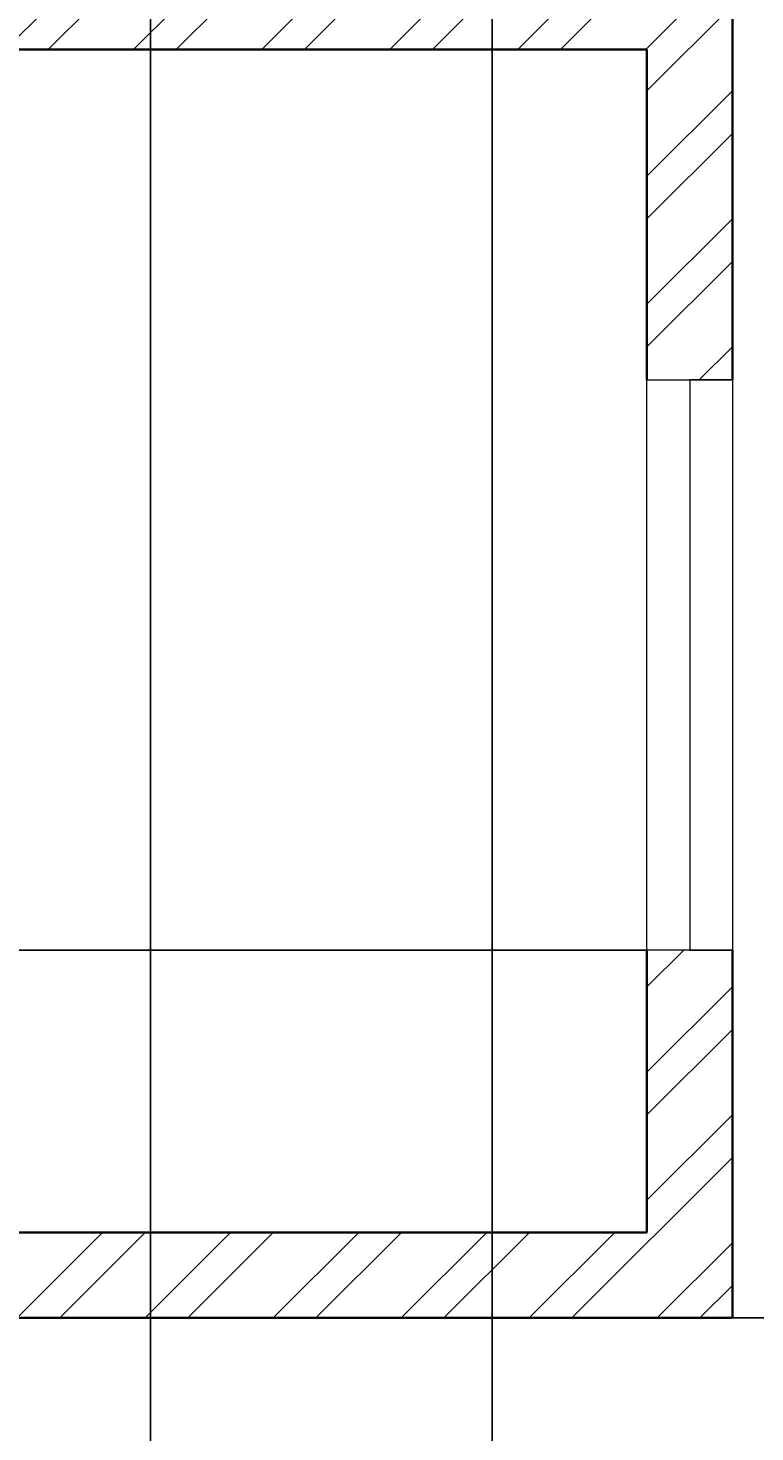
# Model space of a CAD drawing. Units: inches. Extents: x 1748 to 2382, y 1346 to 2284.
# Tile 14 of 26: x 2223 to 2300, y 1456 to 1604. Entities that reach past the tile are written whole.
import ezdxf

# ---------------------------------------------------------------- set-up
doc = ezdxf.new("R2010")
doc.units = ezdxf.units.IN
for name, color, linetype, lineweight in [('A-ANNO-DIMS', 2, 'Continuous', 18), ('A-GLAZ', 191, 'Continuous', 18), ('A-WALL', 7, 'Continuous', 35), ('A-WALL-PATT', 9, 'Continuous', 13)]:
    doc.layers.add(name, color=color, linetype=linetype, lineweight=lineweight)
doc.styles.get("Standard").update_dxf_attribs({"font": 'arial.ttf'})
doc.dimstyles.get("Standard").update_dxf_attribs({"dimtxt": 0.18, "dimasz": 0.18, "dimexe": 0.18, "dimexo": 0.0625, "dimgap": 0.09, "dimtad": 0, "dimtih": 1, "dimtoh": 1, "dimdec": 4, "dimzin": 0, "dimdsep": 46, "dimtxsty": 'Standard', "dimcen": 0.09, "dimadec": 0, "dimazin": 0, "dimtfac": 1, "dimtdec": 4, "dimtofl": 0, "dimtmove": 0, "dimatfit": 3, "dimfxl": 1, "dimtolj": 1, "dimtzin": 0, "dimarcsym": 0})

# ---------------------------------------------------------------- blocks, each defined once
blk = doc.blocks.new('*D35')
at = {"layer": 'A-ANNO-DIMS', "color": 0, "lineweight": -2, "transparency": 16777216}
for p, q in [((2297.52, 2232.85), (2339.54, 2232.85)), ((2339.36, 2232.67), (2339.36, 1850.53)), ((2339.36, 1468.03), (2339.36, 1850.17)), ((2297.52, 1467.85), (2339.54, 1467.85))]:
    blk.add_line(p, q, dxfattribs=at)
at = {"layer": 'A-ANNO-DIMS', "color": 0, "transparency": 16777216}
for points in [[(2339.33, 2232.67), (2339.39, 2232.67), (2339.36, 2232.85)], [(2339.33, 1468.03), (2339.39, 1468.03), (2339.36, 1467.85)]]:
    blk.add_solid(points, dxfattribs=at)
at = {"layer": 'Defpoints', "color": 0, "transparency": 16777216}
for p in [(2297.46, 2232.85), (2339.36, 2232.85), (2297.46, 1467.85)]:
    blk.add_point(p, dxfattribs=at)
at = {"layer": 'A-ANNO-DIMS', "color": 0, "transparency": 16777216, "insert": (2339.36, 1850.35), "char_height": 0.18, "attachment_point": 5}
blk.add_mtext('\\A1;765', dxfattribs=at)
blk = doc.blocks.new('*D49')
at = {"layer": 'A-ANNO-DIMS', "color": 0, "lineweight": -2, "transparency": 16777216}
for p, q in [((2236.23, 1913.29), (2236.23, 1360.47)), ((2272.19, 1913.29), (2272.19, 1360.47)), ((2236.41, 1360.65), (2253.82, 1360.65)), ((2272.01, 1360.65), (2254.61, 1360.65))]:
    blk.add_line(p, q, dxfattribs=at)
at = {"layer": 'A-ANNO-DIMS', "color": 0, "transparency": 16777216}
for points in [[(2236.41, 1360.68), (2236.41, 1360.62), (2236.23, 1360.65)], [(2272.01, 1360.68), (2272.01, 1360.62), (2272.19, 1360.65)]]:
    blk.add_solid(points, dxfattribs=at)
at = {"layer": 'Defpoints', "color": 0, "transparency": 16777216}
for p in [(2236.23, 1913.35), (2272.19, 1913.35), (2272.19, 1360.65)]:
    blk.add_point(p, dxfattribs=at)
at = {"layer": 'A-ANNO-DIMS', "color": 0, "transparency": 16777216, "insert": (2254.21, 1360.65), "char_height": 0.18, "attachment_point": 5}
blk.add_mtext('\\A1;35.96', dxfattribs=at)
blk = doc.blocks.new('*D54')
at = {"layer": 'A-ANNO-DIMS', "color": 0, "lineweight": -2, "transparency": 16777216}
for p, q in [((2288.4, 1506.57), (1779.88, 1506.57)), ((1780.06, 1506.39), (1780.06, 1491.89)), ((1780.06, 1477.03), (1780.06, 1491.53)), ((2288.4, 1476.85), (1779.88, 1476.85))]:
    blk.add_line(p, q, dxfattribs=at)
at = {"layer": 'A-ANNO-DIMS', "color": 0, "transparency": 16777216}
for points in [[(1780.03, 1506.39), (1780.09, 1506.39), (1780.06, 1506.57)], [(1780.03, 1477.03), (1780.09, 1477.03), (1780.06, 1476.85)]]:
    blk.add_solid(points, dxfattribs=at)
at = {"layer": 'Defpoints', "color": 0, "transparency": 16777216}
for p in [(1780.06, 1506.57), (2288.46, 1506.57), (2288.46, 1476.85)]:
    blk.add_point(p, dxfattribs=at)
at = {"layer": 'A-ANNO-DIMS', "color": 0, "transparency": 16777216, "insert": (1780.06, 1491.71), "char_height": 0.18, "attachment_point": 5}
blk.add_mtext('\\A1;29.716', dxfattribs=at)

msp = doc.modelspace()

# ---------------------------------------------------------------- hatches: boundary and pattern name
at = {"layer": 'A-WALL-PATT'}
h = msp.add_hatch(dxfattribs=at)
h.set_pattern_fill('ANSI32', color=256)
h.paths.add_polyline_path([(1919.6777, 1476.8497), (1900.6426, 1476.8497), (1900.6426, 1522.0826), (1898.3926, 1522.0826), (1896.1426, 1522.0826), (1896.1426, 1476.8497), (1857.1426, 1476.8497), (1857.1426, 1467.8497), (1896.1426, 1467.8497), (1919.6777, 1467.8497), (1919.6777, 1472.3497)])
h.paths.add_polyline_path([(2018.7873, 1472.3497), (2018.7873, 1476.8497), (2010.9607, 1476.8497), (2010.9607, 1560.8497), (2034.9607, 1560.8497), (2034.9607, 1565.3497), (2006.4607, 1565.3497), (2006.4607, 1476.8497), (1955.6777, 1476.8497), (1955.6777, 1467.8497), (2018.7873, 1467.8497)])
h.paths.add_polyline_path([(2152.3354, 1472.3497), (2152.3354, 1476.8497), (2115.9607, 1476.8497), (2115.9607, 1565.3497), (2109.2204, 1565.3497), (2109.2204, 1563.0997), (2109.2204, 1560.8497), (2111.4607, 1560.8497), (2111.4607, 1476.8497), (2095.3617, 1476.8497), (2095.3617, 1467.8497), (2152.3354, 1467.8497)])
h.paths.add_polyline_path([(2071.3617, 1476.8497), (2063.4607, 1476.8497), (2063.4607, 1560.8497), (2090.1865, 1560.8497), (2090.1865, 1565.3497), (2063.4607, 1565.3497), (2063.4607, 1572.5485), (2061.2107, 1572.5485), (2058.9607, 1572.5485), (2058.9607, 1565.3497), (2055.6281, 1565.3497), (2055.6281, 1560.8497), (2058.9607, 1560.8497), (2058.9607, 1476.8497), (2042.7873, 1476.8497), (2042.7873, 1467.8497), (2071.3617, 1467.8497), (2071.3617, 1472.3497)])
h.paths.add_polyline_path([(2297.4607, 1506.5652), (2288.4607, 1506.5652), (2288.4607, 1476.8497), (2212.3354, 1476.8497), (2212.3354, 1467.8497), (2297.4607, 1467.8497)])
h.paths.add_polyline_path([(2297.4607, 1645.3038), (2288.4607, 1645.3038), (2288.4607, 1605.8497), (2058.9607, 1605.8497), (2058.9607, 1600.1857), (2061.2107, 1600.1857), (2063.4607, 1600.1857), (2063.4607, 1601.3497), (2288.4607, 1601.3497), (2288.4607, 1566.5652), (2297.4607, 1566.5652)])
h.paths.add_polyline_path([(2010.9607, 1609.0561), (2008.7107, 1609.0561), (2006.4607, 1609.0561), (2006.4607, 1605.8497), (1900.6426, 1605.8497), (1900.6426, 1609.7171), (1898.3926, 1609.7171), (1896.1426, 1609.7171), (1896.1426, 1605.8497), (1857.1426, 1605.8497), (1857.1426, 1601.3497), (1896.1426, 1601.3497), (1896.1426, 1542.5447), (1900.6426, 1542.5447), (1900.6426, 1601.3497), (2010.9607, 1601.3497)])
h.paths.add_polyline_path([(1928.9457, 1401.1212), (2176.8693, 1401.1212), (2176.8693, 1438.214), (1928.9457, 1438.214)], flags=9)
h.paths.add_polyline_path([(2122.2668, 2048.1927), (2177.9387, 2048.1927), (2177.9387, 2066.85), (2122.2668, 2066.85)], flags=9)
h.paths.add_polyline_path([(2272.688, 2153.8197), (2272.688, 2216.746), (2262.3845, 2216.746), (2262.3845, 2153.8197)], flags=9)
h.paths.add_polyline_path([(2157.2928, 2166.5593), (2196.3822, 2166.5593), (2196.3822, 2185.2167), (2157.2928, 2185.2167)], flags=9)
h.paths.add_polyline_path([(2089.3407, 2162.0698), (2124.3987, 2162.0698), (2124.3987, 2180.7272), (2089.3407, 2180.7272)], flags=9)
h.paths.add_polyline_path([(2037.4521, 2160.0913), (2072.5101, 2160.0913), (2072.5101, 2178.7486), (2037.4521, 2178.7486)], flags=9)
h.paths.add_polyline_path([(1884.7894, 2104.1554), (1923.6297, 2104.1554), (1923.6297, 2122.8127), (1884.7894, 2122.8127)], flags=9)
h.paths.add_polyline_path([(1851.2832, 2142.9749), (1851.2832, 2199.3051), (1840.9796, 2199.3051), (1840.9796, 2142.9749)], flags=9)
h.paths.add_polyline_path([(1844.8763, 2017.2834), (1844.8763, 2073.6136), (1834.5728, 2073.6136), (1834.5728, 2017.2834)], flags=9)
h.paths.add_polyline_path([(1897.1577, 2073.1279), (1935.9981, 2073.1279), (1935.9981, 2091.7853), (1897.1577, 2091.7853)], flags=9)
h.paths.add_polyline_path([(1952.3395, 1802.4231), (2008.0114, 1802.4231), (2008.0114, 1821.0805), (1952.3395, 1821.0805)], flags=9)
h.paths.add_polyline_path([(1978.8184, 1857.6841), (2017.7338, 1857.6841), (2017.7338, 1876.3415), (1978.8184, 1876.3415)], flags=9)
h.paths.add_polyline_path([(1979.6513, 1925.9516), (2008.8089, 1925.9516), (2008.8089, 1944.6089), (1979.6513, 1944.6089)], flags=9)
h.paths.add_polyline_path([(1838.5553, 1860.3527), (1877.3957, 1860.3527), (1877.3957, 1879.01), (1838.5553, 1879.01)], flags=9)
h.paths.add_polyline_path([(1883.9018, 1787.3013), (1883.9018, 1843.6315), (1873.5983, 1843.6315), (1873.5983, 1787.3013)], flags=9)
h.paths.add_polyline_path([(1873.7079, 1509.1938), (1873.7079, 1583.7709), (1863.4044, 1583.7709), (1863.4044, 1509.1938)], flags=9)
h.paths.add_polyline_path([(1916.2259, 1603.3681), (1955.0663, 1603.3681), (1955.0663, 1622.0254), (1916.2259, 1622.0254)], flags=9)
h.paths.add_polyline_path([(1876.3013, 1636.757), (1876.3013, 1693.0871), (1865.9978, 1693.0871), (1865.9978, 1636.757)], flags=9)
h.paths.add_polyline_path([(1921.3138, 1521.8316), (1964.0662, 1521.8316), (1964.0662, 1540.489), (1921.3138, 1540.489)], flags=9)
h.paths.add_polyline_path([(2017.5657, 1497.5078), (2046.7983, 1497.5078), (2046.7983, 1516.1651), (2017.5657, 1516.1651)], flags=9)
h.paths.add_polyline_path([(2066.8661, 1499.3902), (2096.0988, 1499.3902), (2096.0988, 1518.0475), (2066.8661, 1518.0475)], flags=9)
h.paths.add_polyline_path([(2155.4835, 1571.6596), (2198.2358, 1571.6596), (2198.2358, 1590.3169), (2155.4835, 1590.3169)], flags=25)
h.paths.add_polyline_path([(2094.9136, 1664.6812), (2150.5855, 1664.6812), (2150.5855, 1683.3386), (2094.9136, 1683.3386)], flags=9)
h.paths.add_polyline_path([(2257.6902, 1863.1628), (2269.8935, 1863.1628), (2269.8935, 1873.4664), (2257.6902, 1873.4664)], flags=9)
h.paths.add_polyline_path([(2164.0748, 1880.3089), (2189.8694, 1880.3089), (2189.8694, 1890.6124), (2164.0748, 1890.6124)], flags=9)
h.paths.add_polyline_path([(2239.4394, 1931.0585), (2268.8187, 1931.0585), (2268.8187, 1949.7159), (2239.4394, 1949.7159)], flags=9)

# ---------------------------------------------------------------- linework, layer by layer
at = {"layer": 'A-GLAZ'}
for p, q in [((2288.4607, 1566.5652), (2297.4607, 1566.5652)), ((2288.4607, 1506.5652), (2288.4607, 1566.5652)), ((2297.4607, 1566.5652), (2292.9607, 1566.5652)), ((2292.9607, 1566.5652), (2292.9607, 1506.5652)), ((2297.4607, 1566.5652), (2297.4607, 1506.5652)), ((2297.4607, 1506.5652), (2288.4607, 1506.5652)), ((2292.9607, 1506.5652), (2297.4607, 1506.5652))]:
    msp.add_line(p, q, dxfattribs=at)
at = {"layer": 'A-WALL'}
for p, q in [((2297.4607, 1645.3038), (2297.4607, 1566.5652)), ((2063.4607, 1601.3497), (2288.4607, 1601.3497)), ((2288.4607, 1601.3497), (2288.4607, 1566.5652)), ((2288.4607, 1506.5652), (2288.4607, 1476.8497)), ((2297.4607, 1506.5652), (2297.4607, 1467.8497)), ((2212.3354, 1476.8497), (2288.4607, 1476.8497)), ((2212.3354, 1467.8497), (2297.4607, 1467.8497))]:
    msp.add_line(p, q, dxfattribs=at)

# ---------------------------------------------------------------- dimensions: what is measured, and where the dimension line sits
at = {"layer": 'A-ANNO-DIMS'}
for base, p1, p2, override, picture, middle in [((2339.3607, 2232.8497), (2297.4607, 1467.8497), (2297.4607, 2232.8497), {"dimdec": 0, "dimlfac": 1, "dimrnd": 0, "dimzin": 0, "dimdsep": 46, "dimlunit": 2}, '*D35', (2339.3607, 1850.3497)), ((1780.06066, 1506.56516), (2288.46066, 1476.84965), (2288.46066, 1506.56516), {"dimdec": 3, "dimlfac": 1, "dimrnd": 0, "dimzin": 0, "dimdsep": 46, "dimlunit": 2}, '*D54', (1780.06066, 1491.7074))]:
    dim = msp.add_linear_dim(base=base, p1=p1, p2=p2, angle=90, dimstyle='Standard', override=override, dxfattribs=at)
    dim.commit()
    dim.dimension.update_dxf_attribs({"geometry": picture, "text_midpoint": middle})
dim = msp.add_linear_dim(base=(2272.1921, 1360.6451), p1=(2236.234, 1913.3497), p2=(2272.1921, 1913.3497), dimstyle='Standard', override={"dimdec": 2, "dimlfac": 1, "dimrnd": 0, "dimzin": 0, "dimdsep": 46, "dimlunit": 2}, dxfattribs=at)
dim.commit()
dim.dimension.update_dxf_attribs({"geometry": '*D49', "text_midpoint": (2254.213, 1360.6451)})

doc.saveas('drawing.dxf')
